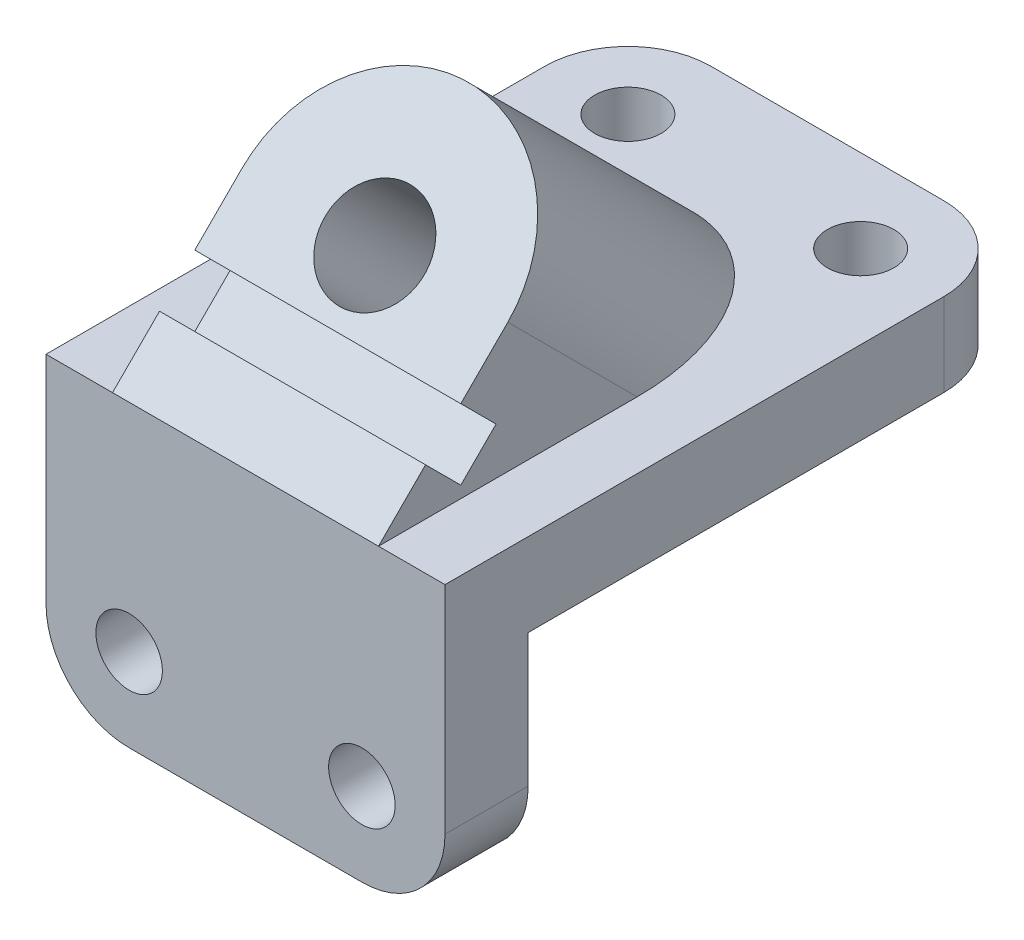
ISO-10303-21;
HEADER;
FILE_DESCRIPTION(('STEP AP214'),'2;1');
FILE_NAME('part.step','',(''),(''),'','','');
FILE_SCHEMA(('AUTOMOTIVE_DESIGN { 1 0 10303 214 1 1 1 1 }'));
ENDSEC;
DATA;
#1=APPLICATION_CONTEXT('core data for automotive mechanical design processes');
#2=APPLICATION_PROTOCOL_DEFINITION('international standard','automotive_design',2000,#1);
#3=PRODUCT_CONTEXT('',#1,'mechanical');
#4=PRODUCT('Part','Part','',(#3));
#5=PRODUCT_RELATED_PRODUCT_CATEGORY('part','',(#4));
#6=PRODUCT_DEFINITION_FORMATION('','',#4);
#7=PRODUCT_DEFINITION_CONTEXT('part definition',#1,'design');
#8=PRODUCT_DEFINITION('design','',#6,#7);
#9=PRODUCT_DEFINITION_SHAPE('','',#8);
#10=(LENGTH_UNIT() NAMED_UNIT(*) SI_UNIT(.MILLI.,.METRE.));
#11=(NAMED_UNIT(*) PLANE_ANGLE_UNIT() SI_UNIT($,.RADIAN.));
#12=(NAMED_UNIT(*) SI_UNIT($,.STERADIAN.) SOLID_ANGLE_UNIT());
#13=UNCERTAINTY_MEASURE_WITH_UNIT(LENGTH_MEASURE(1.E-05),#10,'distance_accuracy_value','');
#14=(GEOMETRIC_REPRESENTATION_CONTEXT(3) GLOBAL_UNCERTAINTY_ASSIGNED_CONTEXT((#13)) GLOBAL_UNIT_ASSIGNED_CONTEXT((#10,
#11,#12)) REPRESENTATION_CONTEXT('',''));
#15=CARTESIAN_POINT('',(0.,0.,0.));
#16=DIRECTION('',(0.,0.,1.));
#17=DIRECTION('',(1.,0.,0.));
#18=AXIS2_PLACEMENT_3D('',#15,#16,#17);
#19=CARTESIAN_POINT('',(60.,0.,0.));
#20=DIRECTION('',(0.,-0.707106781186543,-0.707106781186552));
#21=DIRECTION('',(0.,0.707106781186552,-0.707106781186543));
#22=AXIS2_PLACEMENT_3D('',#19,#20,#21);
#23=PLANE('',#22);
#24=CARTESIAN_POINT('',(0.,38.8908729652603,-38.8908729652599));
#25=DIRECTION('',(0.,0.707106781186543,0.707106781186552));
#26=DIRECTION('',(0.,-0.707106781186552,0.707106781186543));
#27=AXIS2_PLACEMENT_3D('',#24,#25,#26);
#28=CIRCLE('',#27,15.);
#29=CARTESIAN_POINT('',(0.,28.2842712474621,-28.2842712474617));
#30=VERTEX_POINT('',#29);
#31=EDGE_CURVE('E209',#30,#30,#28,.T.);
#32=ORIENTED_EDGE('',*,*,#31,.F.);
#33=EDGE_LOOP('',(#32));
#34=FACE_BOUND('',#33,.T.);
#35=DIRECTION('',(1.,0.,0.));
#36=VECTOR('',#35,1.);
#37=CARTESIAN_POINT('',(-40.,24.7487373415293,-24.748737341529));
#38=LINE('',#37,#36);
#39=CARTESIAN_POINT('',(-40.,24.7487373415293,-24.748737341529));
#40=VERTEX_POINT('',#39);
#41=CARTESIAN_POINT('',(40.,24.7487373415293,-24.748737341529));
#42=VERTEX_POINT('',#41);
#43=EDGE_CURVE('E207',#40,#42,#38,.T.);
#44=ORIENTED_EDGE('',*,*,#43,.T.);
#45=DIRECTION('',(0.,-0.707106781186552,0.707106781186543));
#46=VECTOR('',#45,1.);
#47=CARTESIAN_POINT('',(40.,0.,0.));
#48=LINE('',#47,#46);
#49=CARTESIAN_POINT('',(40.,38.8908729652603,-38.8908729652599));
#50=VERTEX_POINT('',#49);
#51=EDGE_CURVE('E243',#50,#42,#48,.T.);
#52=ORIENTED_EDGE('',*,*,#51,.F.);
#53=CARTESIAN_POINT('',(0.,38.8908729652603,-38.8908729652599));
#54=DIRECTION('',(0.,0.707106781186543,0.707106781186552));
#55=DIRECTION('',(0.,-0.707106781186552,0.707106781186543));
#56=AXIS2_PLACEMENT_3D('',#53,#54,#55);
#57=CIRCLE('',#56,40.);
#58=CARTESIAN_POINT('',(-40.,38.8908729652603,-38.8908729652599));
#59=VERTEX_POINT('',#58);
#60=EDGE_CURVE('E259',#59,#50,#57,.F.);
#61=ORIENTED_EDGE('',*,*,#60,.F.);
#62=DIRECTION('',(0.,0.707106781186552,-0.707106781186543));
#63=VECTOR('',#62,1.);
#64=CARTESIAN_POINT('',(-40.,0.,0.));
#65=LINE('',#64,#63);
#66=EDGE_CURVE('E246',#40,#59,#65,.T.);
#67=ORIENTED_EDGE('',*,*,#66,.F.);
#68=EDGE_LOOP('',(#44,#52,#61,#67));
#69=FACE_BOUND('',#68,.T.);
#70=ADVANCED_FACE('F67',(#34,#69),#23,.F.);
#71=CARTESIAN_POINT('',(-40.,-129.493706197148,-129.49370619715));
#72=DIRECTION('',(1.,0.,0.));
#73=DIRECTION('',(0.,0.,-1.));
#74=AXIS2_PLACEMENT_3D('',#71,#72,#73);
#75=PLANE('',#74);
#76=DIRECTION('',(0.,0.707106781186543,0.707106781186552));
#77=VECTOR('',#76,1.);
#78=CARTESIAN_POINT('',(-40.,14.1421356237312,-35.3553390593273));
#79=LINE('',#78,#77);
#80=CARTESIAN_POINT('',(-40.,14.1421356237312,-35.3553390593273));
#81=VERTEX_POINT('',#80);
#82=EDGE_CURVE('E202',#81,#40,#79,.T.);
#83=ORIENTED_EDGE('',*,*,#82,.T.);
#84=ORIENTED_EDGE('',*,*,#66,.T.);
#85=DIRECTION('',(0.,0.707106781186543,0.707106781186552));
#86=VECTOR('',#85,1.);
#87=CARTESIAN_POINT('',(-40.,-90.602833231888,-168.38457916241));
#88=LINE('',#87,#86);
#89=CARTESIAN_POINT('',(-40.,0.,-77.7817459305207));
#90=VERTEX_POINT('',#89);
#91=EDGE_CURVE('E253',#90,#59,#88,.T.);
#92=ORIENTED_EDGE('',*,*,#91,.F.);
#93=DIRECTION('',(0.,0.,1.));
#94=VECTOR('',#93,1.);
#95=CARTESIAN_POINT('',(-40.,0.,-129.49370619715));
#96=LINE('',#95,#94);
#97=CARTESIAN_POINT('',(-40.,0.,0.));
#98=VERTEX_POINT('',#97);
#99=EDGE_CURVE('E255',#90,#98,#96,.T.);
#100=ORIENTED_EDGE('',*,*,#99,.T.);
#101=CARTESIAN_POINT('',(-40.,14.1421356237311,-14.1421356237309));
#102=VERTEX_POINT('',#101);
#103=EDGE_CURVE('E257',#98,#102,#65,.T.);
#104=ORIENTED_EDGE('',*,*,#103,.T.);
#105=DIRECTION('',(0.,0.707106781186543,0.707106781186552));
#106=VECTOR('',#105,1.);
#107=CARTESIAN_POINT('',(-40.,3.5355339059329,-24.7487373415292));
#108=LINE('',#107,#106);
#109=CARTESIAN_POINT('',(-40.,3.5355339059329,-24.7487373415292));
#110=VERTEX_POINT('',#109);
#111=EDGE_CURVE('E213',#110,#102,#108,.T.);
#112=ORIENTED_EDGE('',*,*,#111,.F.);
#113=DIRECTION('',(0.,0.707106781186552,-0.707106781186543));
#114=VECTOR('',#113,1.);
#115=CARTESIAN_POINT('',(-40.,3.5355339059329,-24.7487373415292));
#116=LINE('',#115,#114);
#117=EDGE_CURVE('E193',#110,#81,#116,.T.);
#118=ORIENTED_EDGE('',*,*,#117,.T.);
#119=EDGE_LOOP('',(#83,#84,#92,#100,#104,#112,#118));
#120=FACE_BOUND('',#119,.T.);
#121=ADVANCED_FACE('F214',(#120),#75,.F.);
#122=CARTESIAN_POINT('',(40.,-129.493706197148,-129.49370619715));
#123=DIRECTION('',(-1.,0.,0.));
#124=DIRECTION('',(0.,-1.,0.));
#125=AXIS2_PLACEMENT_3D('',#122,#123,#124);
#126=PLANE('',#125);
#127=DIRECTION('',(0.,0.707106781186543,0.707106781186552));
#128=VECTOR('',#127,1.);
#129=CARTESIAN_POINT('',(40.,14.1421356237312,-35.3553390593273));
#130=LINE('',#129,#128);
#131=CARTESIAN_POINT('',(40.,14.1421356237312,-35.3553390593273));
#132=VERTEX_POINT('',#131);
#133=EDGE_CURVE('E208',#132,#42,#130,.T.);
#134=ORIENTED_EDGE('',*,*,#133,.F.);
#135=DIRECTION('',(0.,0.707106781186552,-0.707106781186543));
#136=VECTOR('',#135,1.);
#137=CARTESIAN_POINT('',(40.,3.5355339059329,-24.7487373415292));
#138=LINE('',#137,#136);
#139=CARTESIAN_POINT('',(40.,3.5355339059329,-24.7487373415292));
#140=VERTEX_POINT('',#139);
#141=EDGE_CURVE('E198',#140,#132,#138,.T.);
#142=ORIENTED_EDGE('',*,*,#141,.F.);
#143=DIRECTION('',(0.,0.707106781186543,0.707106781186552));
#144=VECTOR('',#143,1.);
#145=CARTESIAN_POINT('',(40.,3.5355339059329,-24.7487373415292));
#146=LINE('',#145,#144);
#147=CARTESIAN_POINT('',(40.,14.142135623731,-14.1421356237309));
#148=VERTEX_POINT('',#147);
#149=EDGE_CURVE('E230',#140,#148,#146,.T.);
#150=ORIENTED_EDGE('',*,*,#149,.T.);
#151=CARTESIAN_POINT('',(40.,0.,0.));
#152=VERTEX_POINT('',#151);
#153=EDGE_CURVE('E245',#148,#152,#48,.T.);
#154=ORIENTED_EDGE('',*,*,#153,.T.);
#155=DIRECTION('',(0.,0.,-1.));
#156=VECTOR('',#155,1.);
#157=CARTESIAN_POINT('',(40.,0.,-129.49370619715));
#158=LINE('',#157,#156);
#159=CARTESIAN_POINT('',(40.,0.,-77.7817459305207));
#160=VERTEX_POINT('',#159);
#161=EDGE_CURVE('E238',#152,#160,#158,.T.);
#162=ORIENTED_EDGE('',*,*,#161,.T.);
#163=DIRECTION('',(0.,0.707106781186543,0.707106781186552));
#164=VECTOR('',#163,1.);
#165=CARTESIAN_POINT('',(40.,-90.602833231888,-168.38457916241));
#166=LINE('',#165,#164);
#167=EDGE_CURVE('E237',#160,#50,#166,.T.);
#168=ORIENTED_EDGE('',*,*,#167,.T.);
#169=ORIENTED_EDGE('',*,*,#51,.T.);
#170=EDGE_LOOP('',(#134,#142,#150,#154,#162,#168,#169));
#171=FACE_BOUND('',#170,.T.);
#172=ADVANCED_FACE('F380',(#171),#126,.F.);
#173=CARTESIAN_POINT('',(60.,-64.9999999999998,-25.));
#174=DIRECTION('',(1.,0.,0.));
#175=DIRECTION('',(0.,1.,0.));
#176=AXIS2_PLACEMENT_3D('',#173,#174,#175);
#177=PLANE('',#176);
#178=DIRECTION('',(0.,0.,-1.));
#179=VECTOR('',#178,1.);
#180=CARTESIAN_POINT('',(60.,-25.,-175.));
#181=LINE('',#180,#179);
#182=CARTESIAN_POINT('',(60.,-25.,-25.));
#183=VERTEX_POINT('',#182);
#184=CARTESIAN_POINT('',(60.,-25.,-150.));
#185=VERTEX_POINT('',#184);
#186=EDGE_CURVE('E280',#183,#185,#181,.T.);
#187=ORIENTED_EDGE('',*,*,#186,.T.);
#188=DIRECTION('',(0.,1.,0.));
#189=VECTOR('',#188,1.);
#190=CARTESIAN_POINT('',(60.,0.,-150.));
#191=LINE('',#190,#189);
#192=CARTESIAN_POINT('',(60.,0.,-150.));
#193=VERTEX_POINT('',#192);
#194=EDGE_CURVE('E12',#185,#193,#191,.T.);
#195=ORIENTED_EDGE('',*,*,#194,.T.);
#196=DIRECTION('',(0.,0.,1.));
#197=VECTOR('',#196,1.);
#198=CARTESIAN_POINT('',(60.,0.,-25.));
#199=LINE('',#198,#197);
#200=CARTESIAN_POINT('',(60.,0.,0.));
#201=VERTEX_POINT('',#200);
#202=EDGE_CURVE('E304',#193,#201,#199,.T.);
#203=ORIENTED_EDGE('',*,*,#202,.T.);
#204=DIRECTION('',(0.,1.,0.));
#205=VECTOR('',#204,1.);
#206=CARTESIAN_POINT('',(60.,-64.9999999999998,0.));
#207=LINE('',#206,#205);
#208=CARTESIAN_POINT('',(60.,-65.,0.));
#209=VERTEX_POINT('',#208);
#210=EDGE_CURVE('E290',#209,#201,#207,.T.);
#211=ORIENTED_EDGE('',*,*,#210,.F.);
#212=DIRECTION('',(0.,0.,1.));
#213=VECTOR('',#212,1.);
#214=CARTESIAN_POINT('',(60.,-65.,-25.));
#215=LINE('',#214,#213);
#216=CARTESIAN_POINT('',(60.,-65.,-25.));
#217=VERTEX_POINT('',#216);
#218=EDGE_CURVE('E324',#217,#209,#215,.T.);
#219=ORIENTED_EDGE('',*,*,#218,.F.);
#220=DIRECTION('',(0.,1.,0.));
#221=VECTOR('',#220,1.);
#222=CARTESIAN_POINT('',(60.,-64.9999999999998,-25.));
#223=LINE('',#222,#221);
#224=EDGE_CURVE('E286',#217,#183,#223,.T.);
#225=ORIENTED_EDGE('',*,*,#224,.T.);
#226=EDGE_LOOP('',(#187,#195,#203,#211,#219,#225));
#227=FACE_BOUND('',#226,.T.);
#228=ADVANCED_FACE('F381',(#227),#177,.T.);
#229=CARTESIAN_POINT('',(-60.,-64.9999999999998,-25.));
#230=DIRECTION('',(-1.,0.,0.));
#231=DIRECTION('',(0.,0.,1.));
#232=AXIS2_PLACEMENT_3D('',#229,#230,#231);
#233=PLANE('',#232);
#234=DIRECTION('',(0.,0.,1.));
#235=VECTOR('',#234,1.);
#236=CARTESIAN_POINT('',(-60.,0.,-25.));
#237=LINE('',#236,#235);
#238=CARTESIAN_POINT('',(-60.,0.,-150.));
#239=VERTEX_POINT('',#238);
#240=CARTESIAN_POINT('',(-60.,0.,0.));
#241=VERTEX_POINT('',#240);
#242=EDGE_CURVE('E334',#239,#241,#237,.T.);
#243=ORIENTED_EDGE('',*,*,#242,.F.);
#244=DIRECTION('',(0.,1.,0.));
#245=VECTOR('',#244,1.);
#246=CARTESIAN_POINT('',(-60.,-25.,-150.));
#247=LINE('',#246,#245);
#248=CARTESIAN_POINT('',(-60.,-25.,-150.));
#249=VERTEX_POINT('',#248);
#250=EDGE_CURVE('E94',#239,#249,#247,.F.);
#251=ORIENTED_EDGE('',*,*,#250,.T.);
#252=DIRECTION('',(0.,0.,-1.));
#253=VECTOR('',#252,1.);
#254=CARTESIAN_POINT('',(-60.,-25.,-175.));
#255=LINE('',#254,#253);
#256=CARTESIAN_POINT('',(-60.,-25.,-25.));
#257=VERTEX_POINT('',#256);
#258=EDGE_CURVE('E267',#257,#249,#255,.T.);
#259=ORIENTED_EDGE('',*,*,#258,.F.);
#260=DIRECTION('',(0.,-1.,0.));
#261=VECTOR('',#260,1.);
#262=CARTESIAN_POINT('',(-60.,-64.9999999999998,-25.));
#263=LINE('',#262,#261);
#264=CARTESIAN_POINT('',(-60.,-64.9999999999998,-25.));
#265=VERTEX_POINT('',#264);
#266=EDGE_CURVE('E291',#257,#265,#263,.T.);
#267=ORIENTED_EDGE('',*,*,#266,.T.);
#268=DIRECTION('',(0.,0.,1.));
#269=VECTOR('',#268,1.);
#270=CARTESIAN_POINT('',(-60.,-64.9999999999998,-25.));
#271=LINE('',#270,#269);
#272=CARTESIAN_POINT('',(-60.,-64.9999999999998,0.));
#273=VERTEX_POINT('',#272);
#274=EDGE_CURVE('E329',#265,#273,#271,.T.);
#275=ORIENTED_EDGE('',*,*,#274,.T.);
#276=DIRECTION('',(0.,-1.,0.));
#277=VECTOR('',#276,1.);
#278=CARTESIAN_POINT('',(-60.,-64.9999999999998,0.));
#279=LINE('',#278,#277);
#280=EDGE_CURVE('E315',#241,#273,#279,.T.);
#281=ORIENTED_EDGE('',*,*,#280,.F.);
#282=EDGE_LOOP('',(#243,#251,#259,#267,#275,#281));
#283=FACE_BOUND('',#282,.T.);
#284=ADVANCED_FACE('F357',(#283),#233,.T.);
#285=CARTESIAN_POINT('',(35.,-65.,-25.));
#286=DIRECTION('',(0.,0.,1.));
#287=DIRECTION('',(1.,0.,0.));
#288=AXIS2_PLACEMENT_3D('',#285,#286,#287);
#289=CYLINDRICAL_SURFACE('',#288,25.);
#290=CARTESIAN_POINT('',(35.,-65.,0.));
#291=DIRECTION('',(0.,0.,1.));
#292=DIRECTION('',(1.,0.,0.));
#293=AXIS2_PLACEMENT_3D('',#290,#291,#292);
#294=CIRCLE('',#293,25.);
#295=CARTESIAN_POINT('',(34.9999999999999,-90.,0.));
#296=VERTEX_POINT('',#295);
#297=EDGE_CURVE('E295',#296,#209,#294,.T.);
#298=ORIENTED_EDGE('',*,*,#297,.F.);
#299=DIRECTION('',(0.,0.,1.));
#300=VECTOR('',#299,1.);
#301=CARTESIAN_POINT('',(34.9999999999999,-90.,-25.));
#302=LINE('',#301,#300);
#303=CARTESIAN_POINT('',(34.9999999999999,-90.,-25.));
#304=VERTEX_POINT('',#303);
#305=EDGE_CURVE('E326',#304,#296,#302,.T.);
#306=ORIENTED_EDGE('',*,*,#305,.F.);
#307=CARTESIAN_POINT('',(35.,-65.,-25.));
#308=DIRECTION('',(0.,0.,1.));
#309=DIRECTION('',(1.,0.,0.));
#310=AXIS2_PLACEMENT_3D('',#307,#308,#309);
#311=CIRCLE('',#310,25.);
#312=EDGE_CURVE('E305',#304,#217,#311,.T.);
#313=ORIENTED_EDGE('',*,*,#312,.T.);
#314=ORIENTED_EDGE('',*,*,#218,.T.);
#315=EDGE_LOOP('',(#298,#306,#313,#314));
#316=FACE_BOUND('',#315,.T.);
#317=ADVANCED_FACE('F439',(#316),#289,.T.);
#318=CARTESIAN_POINT('',(-34.9999999999998,-90.,-25.));
#319=DIRECTION('',(0.,-1.,0.));
#320=DIRECTION('',(1.,0.,0.));
#321=AXIS2_PLACEMENT_3D('',#318,#319,#320);
#322=PLANE('',#321);
#323=DIRECTION('',(1.,0.,0.));
#324=VECTOR('',#323,1.);
#325=CARTESIAN_POINT('',(-34.9999999999998,-90.,0.));
#326=LINE('',#325,#324);
#327=CARTESIAN_POINT('',(-34.9999999999998,-90.,0.));
#328=VERTEX_POINT('',#327);
#329=EDGE_CURVE('E319',#328,#296,#326,.T.);
#330=ORIENTED_EDGE('',*,*,#329,.F.);
#331=DIRECTION('',(0.,0.,1.));
#332=VECTOR('',#331,1.);
#333=CARTESIAN_POINT('',(-34.9999999999998,-90.,-25.));
#334=LINE('',#333,#332);
#335=CARTESIAN_POINT('',(-34.9999999999998,-90.,-25.));
#336=VERTEX_POINT('',#335);
#337=EDGE_CURVE('E328',#336,#328,#334,.T.);
#338=ORIENTED_EDGE('',*,*,#337,.F.);
#339=DIRECTION('',(1.,0.,0.));
#340=VECTOR('',#339,1.);
#341=CARTESIAN_POINT('',(-34.9999999999998,-90.,-25.));
#342=LINE('',#341,#340);
#343=EDGE_CURVE('E299',#336,#304,#342,.T.);
#344=ORIENTED_EDGE('',*,*,#343,.T.);
#345=ORIENTED_EDGE('',*,*,#305,.T.);
#346=EDGE_LOOP('',(#330,#338,#344,#345));
#347=FACE_BOUND('',#346,.T.);
#348=ADVANCED_FACE('F442',(#347),#322,.T.);
#349=CARTESIAN_POINT('',(-35.,-65.,-25.));
#350=DIRECTION('',(0.,0.,1.));
#351=DIRECTION('',(1.,0.,0.));
#352=AXIS2_PLACEMENT_3D('',#349,#350,#351);
#353=CYLINDRICAL_SURFACE('',#352,25.);
#354=CARTESIAN_POINT('',(-35.,-65.,0.));
#355=DIRECTION('',(0.,0.,1.));
#356=DIRECTION('',(-1.,0.,0.));
#357=AXIS2_PLACEMENT_3D('',#354,#355,#356);
#358=CIRCLE('',#357,25.);
#359=EDGE_CURVE('E314',#273,#328,#358,.T.);
#360=ORIENTED_EDGE('',*,*,#359,.F.);
#361=ORIENTED_EDGE('',*,*,#274,.F.);
#362=CARTESIAN_POINT('',(-35.,-65.,-25.));
#363=DIRECTION('',(0.,0.,1.));
#364=DIRECTION('',(-1.,0.,0.));
#365=AXIS2_PLACEMENT_3D('',#362,#363,#364);
#366=CIRCLE('',#365,25.);
#367=EDGE_CURVE('E298',#265,#336,#366,.T.);
#368=ORIENTED_EDGE('',*,*,#367,.T.);
#369=ORIENTED_EDGE('',*,*,#337,.T.);
#370=EDGE_LOOP('',(#360,#361,#368,#369));
#371=FACE_BOUND('',#370,.T.);
#372=ADVANCED_FACE('F450',(#371),#353,.T.);
#373=CARTESIAN_POINT('',(-60.,0.,-25.));
#374=DIRECTION('',(0.,1.,0.));
#375=DIRECTION('',(-1.,0.,0.));
#376=AXIS2_PLACEMENT_3D('',#373,#374,#375);
#377=PLANE('',#376);
#378=CARTESIAN_POINT('',(-35.,0.,-150.));
#379=DIRECTION('',(0.,1.,0.));
#380=DIRECTION('',(-1.,0.,0.));
#381=AXIS2_PLACEMENT_3D('',#378,#379,#380);
#382=CIRCLE('',#381,10.);
#383=CARTESIAN_POINT('',(-45.,0.,-150.));
#384=VERTEX_POINT('',#383);
#385=EDGE_CURVE('E477',#384,#384,#382,.T.);
#386=ORIENTED_EDGE('',*,*,#385,.F.);
#387=EDGE_LOOP('',(#386));
#388=FACE_BOUND('',#387,.T.);
#389=CARTESIAN_POINT('',(35.,0.,-150.));
#390=DIRECTION('',(0.,1.,0.));
#391=DIRECTION('',(-1.,0.,0.));
#392=AXIS2_PLACEMENT_3D('',#389,#390,#391);
#393=CIRCLE('',#392,10.);
#394=CARTESIAN_POINT('',(25.,0.,-150.));
#395=VERTEX_POINT('',#394);
#396=EDGE_CURVE('E485',#395,#395,#393,.T.);
#397=ORIENTED_EDGE('',*,*,#396,.F.);
#398=EDGE_LOOP('',(#397));
#399=FACE_BOUND('',#398,.T.);
#400=DIRECTION('',(-1.,0.,0.));
#401=VECTOR('',#400,1.);
#402=CARTESIAN_POINT('',(60.,0.,-175.));
#403=LINE('',#402,#401);
#404=CARTESIAN_POINT('',(35.,0.,-175.));
#405=VERTEX_POINT('',#404);
#406=CARTESIAN_POINT('',(-35.,0.,-175.));
#407=VERTEX_POINT('',#406);
#408=EDGE_CURVE('E276',#405,#407,#403,.T.);
#409=ORIENTED_EDGE('',*,*,#408,.T.);
#410=CARTESIAN_POINT('',(-35.,0.,-150.));
#411=DIRECTION('',(0.,1.,0.));
#412=DIRECTION('',(-1.,0.,0.));
#413=AXIS2_PLACEMENT_3D('',#410,#411,#412);
#414=CIRCLE('',#413,25.);
#415=EDGE_CURVE('E342',#407,#239,#414,.T.);
#416=ORIENTED_EDGE('',*,*,#415,.T.);
#417=ORIENTED_EDGE('',*,*,#242,.T.);
#418=DIRECTION('',(1.,0.,0.));
#419=VECTOR('',#418,1.);
#420=CARTESIAN_POINT('',(0.,0.,0.));
#421=LINE('',#420,#419);
#422=EDGE_CURVE('E258',#241,#98,#421,.T.);
#423=ORIENTED_EDGE('',*,*,#422,.T.);
#424=ORIENTED_EDGE('',*,*,#99,.F.);
#425=CARTESIAN_POINT('',(0.,0.,-77.7817459305207));
#426=DIRECTION('',(0.,1.,0.));
#427=DIRECTION('',(0.,0.,1.));
#428=AXIS2_PLACEMENT_3D('',#425,#426,#427);
#429=ELLIPSE('',#428,56.5685424949241,40.);
#430=EDGE_CURVE('E248',#160,#90,#429,.T.);
#431=ORIENTED_EDGE('',*,*,#430,.F.);
#432=ORIENTED_EDGE('',*,*,#161,.F.);
#433=DIRECTION('',(-1.,0.,0.));
#434=VECTOR('',#433,1.);
#435=CARTESIAN_POINT('',(-60.,0.,0.));
#436=LINE('',#435,#434);
#437=EDGE_CURVE('E307',#201,#152,#436,.T.);
#438=ORIENTED_EDGE('',*,*,#437,.F.);
#439=ORIENTED_EDGE('',*,*,#202,.F.);
#440=CARTESIAN_POINT('',(35.,0.,-150.));
#441=DIRECTION('',(0.,1.,0.));
#442=DIRECTION('',(-1.,0.,0.));
#443=AXIS2_PLACEMENT_3D('',#440,#441,#442);
#444=CIRCLE('',#443,25.);
#445=EDGE_CURVE('E339',#193,#405,#444,.T.);
#446=ORIENTED_EDGE('',*,*,#445,.T.);
#447=EDGE_LOOP('',(#409,#416,#417,#423,#424,#431,#432,#438,#439,#446));
#448=FACE_BOUND('',#447,.T.);
#449=ADVANCED_FACE('F355',(#388,#399,#448),#377,.T.);
#450=CARTESIAN_POINT('',(-35.,-65.,-25.));
#451=DIRECTION('',(0.,0.,-1.));
#452=DIRECTION('',(-1.,0.,0.));
#453=AXIS2_PLACEMENT_3D('',#450,#451,#452);
#454=PLANE('',#453);
#455=CARTESIAN_POINT('',(-35.,-65.,-25.));
#456=DIRECTION('',(0.,0.,-1.));
#457=DIRECTION('',(-1.,0.,0.));
#458=AXIS2_PLACEMENT_3D('',#455,#456,#457);
#459=CIRCLE('',#458,10.);
#460=CARTESIAN_POINT('',(-45.,-65.,-25.));
#461=VERTEX_POINT('',#460);
#462=EDGE_CURVE('E270',#461,#461,#459,.F.);
#463=ORIENTED_EDGE('',*,*,#462,.T.);
#464=EDGE_LOOP('',(#463));
#465=FACE_BOUND('',#464,.T.);
#466=CARTESIAN_POINT('',(35.,-65.,-25.));
#467=DIRECTION('',(0.,0.,-1.));
#468=DIRECTION('',(-1.,0.,0.));
#469=AXIS2_PLACEMENT_3D('',#466,#467,#468);
#470=CIRCLE('',#469,10.);
#471=CARTESIAN_POINT('',(25.,-65.,-25.));
#472=VERTEX_POINT('',#471);
#473=EDGE_CURVE('E252',#472,#472,#470,.F.);
#474=ORIENTED_EDGE('',*,*,#473,.T.);
#475=EDGE_LOOP('',(#474));
#476=FACE_BOUND('',#475,.T.);
#477=DIRECTION('',(-1.,0.,0.));
#478=VECTOR('',#477,1.);
#479=CARTESIAN_POINT('',(60.,-25.,-25.));
#480=LINE('',#479,#478);
#481=EDGE_CURVE('E288',#183,#257,#480,.T.);
#482=ORIENTED_EDGE('',*,*,#481,.F.);
#483=ORIENTED_EDGE('',*,*,#224,.F.);
#484=ORIENTED_EDGE('',*,*,#312,.F.);
#485=ORIENTED_EDGE('',*,*,#343,.F.);
#486=ORIENTED_EDGE('',*,*,#367,.F.);
#487=ORIENTED_EDGE('',*,*,#266,.F.);
#488=EDGE_LOOP('',(#482,#483,#484,#485,#486,#487));
#489=FACE_BOUND('',#488,.T.);
#490=ADVANCED_FACE('F432',(#465,#476,#489),#454,.T.);
#491=CARTESIAN_POINT('',(-35.,-65.,0.));
#492=DIRECTION('',(0.,0.,-1.));
#493=DIRECTION('',(-1.,0.,0.));
#494=AXIS2_PLACEMENT_3D('',#491,#492,#493);
#495=PLANE('',#494);
#496=CARTESIAN_POINT('',(-35.,-65.,0.));
#497=DIRECTION('',(0.,0.,1.));
#498=DIRECTION('',(1.,0.,0.));
#499=AXIS2_PLACEMENT_3D('',#496,#497,#498);
#500=CIRCLE('',#499,10.);
#501=CARTESIAN_POINT('',(-25.,-65.,0.));
#502=VERTEX_POINT('',#501);
#503=EDGE_CURVE('E264',#502,#502,#500,.T.);
#504=ORIENTED_EDGE('',*,*,#503,.F.);
#505=EDGE_LOOP('',(#504));
#506=FACE_BOUND('',#505,.T.);
#507=CARTESIAN_POINT('',(35.,-65.,0.));
#508=DIRECTION('',(0.,0.,1.));
#509=DIRECTION('',(1.,0.,0.));
#510=AXIS2_PLACEMENT_3D('',#507,#508,#509);
#511=CIRCLE('',#510,10.);
#512=CARTESIAN_POINT('',(45.,-65.,0.));
#513=VERTEX_POINT('',#512);
#514=EDGE_CURVE('E275',#513,#513,#511,.T.);
#515=ORIENTED_EDGE('',*,*,#514,.F.);
#516=EDGE_LOOP('',(#515));
#517=FACE_BOUND('',#516,.T.);
#518=ORIENTED_EDGE('',*,*,#210,.T.);
#519=ORIENTED_EDGE('',*,*,#437,.T.);
#520=EDGE_CURVE('E308',#152,#98,#436,.T.);
#521=ORIENTED_EDGE('',*,*,#520,.T.);
#522=ORIENTED_EDGE('',*,*,#422,.F.);
#523=ORIENTED_EDGE('',*,*,#280,.T.);
#524=ORIENTED_EDGE('',*,*,#359,.T.);
#525=ORIENTED_EDGE('',*,*,#329,.T.);
#526=ORIENTED_EDGE('',*,*,#297,.T.);
#527=EDGE_LOOP('',(#518,#519,#521,#522,#523,#524,#525,#526));
#528=FACE_BOUND('',#527,.T.);
#529=ADVANCED_FACE('F363',(#506,#517,#528),#495,.F.);
#530=CARTESIAN_POINT('',(60.,-25.,-175.));
#531=DIRECTION('',(0.,1.,0.));
#532=DIRECTION('',(0.,0.,1.));
#533=AXIS2_PLACEMENT_3D('',#530,#531,#532);
#534=PLANE('',#533);
#535=CARTESIAN_POINT('',(-35.,-25.,-150.));
#536=DIRECTION('',(0.,1.,0.));
#537=DIRECTION('',(0.,0.,1.));
#538=AXIS2_PLACEMENT_3D('',#535,#536,#537);
#539=CIRCLE('',#538,10.);
#540=CARTESIAN_POINT('',(-45.,-25.,-150.));
#541=VERTEX_POINT('',#540);
#542=EDGE_CURVE('E228',#541,#541,#539,.F.);
#543=ORIENTED_EDGE('',*,*,#542,.F.);
#544=EDGE_LOOP('',(#543));
#545=FACE_BOUND('',#544,.T.);
#546=CARTESIAN_POINT('',(35.,-25.,-150.));
#547=DIRECTION('',(0.,1.,0.));
#548=DIRECTION('',(0.,0.,1.));
#549=AXIS2_PLACEMENT_3D('',#546,#547,#548);
#550=CIRCLE('',#549,10.);
#551=CARTESIAN_POINT('',(25.,-25.,-150.));
#552=VERTEX_POINT('',#551);
#553=EDGE_CURVE('E219',#552,#552,#550,.F.);
#554=ORIENTED_EDGE('',*,*,#553,.F.);
#555=EDGE_LOOP('',(#554));
#556=FACE_BOUND('',#555,.T.);
#557=CARTESIAN_POINT('',(0.,-25.,-102.781745930521));
#558=DIRECTION('',(0.,1.,0.));
#559=DIRECTION('',(0.,0.,1.));
#560=AXIS2_PLACEMENT_3D('',#557,#558,#559);
#561=ELLIPSE('',#560,21.2132034355965,15.);
#562=CARTESIAN_POINT('',(0.,-25.,-81.5685424949245));
#563=VERTEX_POINT('',#562);
#564=EDGE_CURVE('E232',#563,#563,#561,.F.);
#565=ORIENTED_EDGE('',*,*,#564,.F.);
#566=EDGE_LOOP('',(#565));
#567=FACE_BOUND('',#566,.T.);
#568=ORIENTED_EDGE('',*,*,#258,.T.);
#569=CARTESIAN_POINT('',(-35.,-25.,-150.));
#570=DIRECTION('',(0.,1.,0.));
#571=DIRECTION('',(0.,0.,1.));
#572=AXIS2_PLACEMENT_3D('',#569,#570,#571);
#573=CIRCLE('',#572,25.);
#574=CARTESIAN_POINT('',(-35.,-25.,-175.));
#575=VERTEX_POINT('',#574);
#576=EDGE_CURVE('E80',#249,#575,#573,.F.);
#577=ORIENTED_EDGE('',*,*,#576,.T.);
#578=DIRECTION('',(-1.,0.,0.));
#579=VECTOR('',#578,1.);
#580=CARTESIAN_POINT('',(60.,-25.,-175.));
#581=LINE('',#580,#579);
#582=CARTESIAN_POINT('',(35.,-25.,-175.));
#583=VERTEX_POINT('',#582);
#584=EDGE_CURVE('E283',#583,#575,#581,.T.);
#585=ORIENTED_EDGE('',*,*,#584,.F.);
#586=CARTESIAN_POINT('',(35.,-25.,-150.));
#587=DIRECTION('',(0.,1.,0.));
#588=DIRECTION('',(0.,0.,1.));
#589=AXIS2_PLACEMENT_3D('',#586,#587,#588);
#590=CIRCLE('',#589,25.);
#591=EDGE_CURVE('E81',#583,#185,#590,.F.);
#592=ORIENTED_EDGE('',*,*,#591,.T.);
#593=ORIENTED_EDGE('',*,*,#186,.F.);
#594=ORIENTED_EDGE('',*,*,#481,.T.);
#595=EDGE_LOOP('',(#568,#577,#585,#592,#593,#594));
#596=FACE_BOUND('',#595,.T.);
#597=ADVANCED_FACE('F343',(#545,#556,#567,#596),#534,.F.);
#598=CARTESIAN_POINT('',(60.,0.,-175.));
#599=DIRECTION('',(0.,0.,1.));
#600=DIRECTION('',(1.,0.,0.));
#601=AXIS2_PLACEMENT_3D('',#598,#599,#600);
#602=PLANE('',#601);
#603=ORIENTED_EDGE('',*,*,#584,.T.);
#604=DIRECTION('',(0.,1.,0.));
#605=VECTOR('',#604,1.);
#606=CARTESIAN_POINT('',(-35.,0.,-175.));
#607=LINE('',#606,#605);
#608=EDGE_CURVE('E337',#575,#407,#607,.T.);
#609=ORIENTED_EDGE('',*,*,#608,.T.);
#610=ORIENTED_EDGE('',*,*,#408,.F.);
#611=DIRECTION('',(0.,1.,0.));
#612=VECTOR('',#611,1.);
#613=CARTESIAN_POINT('',(35.,-25.,-175.));
#614=LINE('',#613,#612);
#615=EDGE_CURVE('E323',#405,#583,#614,.F.);
#616=ORIENTED_EDGE('',*,*,#615,.T.);
#617=EDGE_LOOP('',(#603,#609,#610,#616));
#618=FACE_BOUND('',#617,.T.);
#619=ADVANCED_FACE('F347',(#618),#602,.F.);
#620=CARTESIAN_POINT('',(35.,-65.,-175.001));
#621=DIRECTION('',(0.,0.,1.));
#622=DIRECTION('',(1.,0.,0.));
#623=AXIS2_PLACEMENT_3D('',#620,#621,#622);
#624=CYLINDRICAL_SURFACE('',#623,10.);
#625=ORIENTED_EDGE('',*,*,#473,.F.);
#626=EDGE_LOOP('',(#625));
#627=FACE_BOUND('',#626,.T.);
#628=ORIENTED_EDGE('',*,*,#514,.T.);
#629=EDGE_LOOP('',(#628));
#630=FACE_BOUND('',#629,.T.);
#631=ADVANCED_FACE('F417',(#627,#630),#624,.F.);
#632=CARTESIAN_POINT('',(-35.,-65.,-175.001));
#633=DIRECTION('',(0.,0.,1.));
#634=DIRECTION('',(1.,0.,0.));
#635=AXIS2_PLACEMENT_3D('',#632,#633,#634);
#636=CYLINDRICAL_SURFACE('',#635,10.);
#637=ORIENTED_EDGE('',*,*,#462,.F.);
#638=EDGE_LOOP('',(#637));
#639=FACE_BOUND('',#638,.T.);
#640=ORIENTED_EDGE('',*,*,#503,.T.);
#641=EDGE_LOOP('',(#640));
#642=FACE_BOUND('',#641,.T.);
#643=ADVANCED_FACE('F406',(#639,#642),#636,.F.);
#644=ORIENTED_EDGE('',*,*,#153,.F.);
#645=DIRECTION('',(1.,0.,0.));
#646=VECTOR('',#645,1.);
#647=CARTESIAN_POINT('',(-40.,14.1421356237311,-14.1421356237309));
#648=LINE('',#647,#646);
#649=EDGE_CURVE('E216',#102,#148,#648,.T.);
#650=ORIENTED_EDGE('',*,*,#649,.F.);
#651=ORIENTED_EDGE('',*,*,#103,.F.);
#652=ORIENTED_EDGE('',*,*,#520,.F.);
#653=EDGE_LOOP('',(#644,#650,#651,#652));
#654=FACE_BOUND('',#653,.T.);
#655=ADVANCED_FACE('F368',(#654),#23,.F.);
#656=CARTESIAN_POINT('',(0.,-90.602833231888,-168.38457916241));
#657=DIRECTION('',(0.,0.707106781186543,0.707106781186552));
#658=DIRECTION('',(0.,-0.707106781186552,0.707106781186543));
#659=AXIS2_PLACEMENT_3D('',#656,#657,#658);
#660=CYLINDRICAL_SURFACE('',#659,40.);
#661=ORIENTED_EDGE('',*,*,#430,.T.);
#662=ORIENTED_EDGE('',*,*,#91,.T.);
#663=ORIENTED_EDGE('',*,*,#60,.T.);
#664=ORIENTED_EDGE('',*,*,#167,.F.);
#665=EDGE_LOOP('',(#661,#662,#663,#664));
#666=FACE_BOUND('',#665,.T.);
#667=ADVANCED_FACE('F375',(#666),#660,.T.);
#668=CARTESIAN_POINT('',(0.,-93.6101270347391,-171.391872965261));
#669=DIRECTION('',(0.,0.707106781186543,0.707106781186552));
#670=DIRECTION('',(0.,-0.707106781186552,0.707106781186543));
#671=AXIS2_PLACEMENT_3D('',#668,#669,#670);
#672=CYLINDRICAL_SURFACE('',#671,15.);
#673=ORIENTED_EDGE('',*,*,#31,.T.);
#674=EDGE_LOOP('',(#673));
#675=FACE_BOUND('',#674,.T.);
#676=ORIENTED_EDGE('',*,*,#564,.T.);
#677=EDGE_LOOP('',(#676));
#678=FACE_BOUND('',#677,.T.);
#679=ADVANCED_FACE('F414',(#675,#678),#672,.F.);
#680=CARTESIAN_POINT('',(-40.,14.1421356237312,-35.3553390593273));
#681=DIRECTION('',(0.,-0.707106781186552,0.707106781186543));
#682=DIRECTION('',(0.,-0.707106781186543,-0.707106781186552));
#683=AXIS2_PLACEMENT_3D('',#680,#681,#682);
#684=PLANE('',#683);
#685=ORIENTED_EDGE('',*,*,#43,.F.);
#686=ORIENTED_EDGE('',*,*,#82,.F.);
#687=DIRECTION('',(1.,0.,0.));
#688=VECTOR('',#687,1.);
#689=CARTESIAN_POINT('',(-40.,14.1421356237312,-35.3553390593273));
#690=LINE('',#689,#688);
#691=EDGE_CURVE('E192',#81,#132,#690,.T.);
#692=ORIENTED_EDGE('',*,*,#691,.T.);
#693=ORIENTED_EDGE('',*,*,#133,.T.);
#694=EDGE_LOOP('',(#685,#686,#692,#693));
#695=FACE_BOUND('',#694,.T.);
#696=ADVANCED_FACE('F205',(#695),#684,.T.);
#697=CARTESIAN_POINT('',(-40.,3.5355339059329,-24.7487373415292));
#698=DIRECTION('',(0.,-0.707106781186552,0.707106781186543));
#699=DIRECTION('',(0.,-0.707106781186543,-0.707106781186552));
#700=AXIS2_PLACEMENT_3D('',#697,#698,#699);
#701=PLANE('',#700);
#702=ORIENTED_EDGE('',*,*,#649,.T.);
#703=ORIENTED_EDGE('',*,*,#149,.F.);
#704=DIRECTION('',(1.,0.,0.));
#705=VECTOR('',#704,1.);
#706=CARTESIAN_POINT('',(-40.,3.5355339059329,-24.7487373415292));
#707=LINE('',#706,#705);
#708=EDGE_CURVE('E225',#110,#140,#707,.T.);
#709=ORIENTED_EDGE('',*,*,#708,.F.);
#710=ORIENTED_EDGE('',*,*,#111,.T.);
#711=EDGE_LOOP('',(#702,#703,#709,#710));
#712=FACE_BOUND('',#711,.T.);
#713=ADVANCED_FACE('F470',(#712),#701,.F.);
#714=CARTESIAN_POINT('',(0.,-10.6066017177982,-10.6066017177983));
#715=DIRECTION('',(0.,-0.707106781186543,-0.707106781186552));
#716=DIRECTION('',(0.,0.707106781186552,-0.707106781186543));
#717=AXIS2_PLACEMENT_3D('',#714,#715,#716);
#718=PLANE('',#717);
#719=ORIENTED_EDGE('',*,*,#117,.F.);
#720=ORIENTED_EDGE('',*,*,#708,.T.);
#721=ORIENTED_EDGE('',*,*,#141,.T.);
#722=ORIENTED_EDGE('',*,*,#691,.F.);
#723=EDGE_LOOP('',(#719,#720,#721,#722));
#724=FACE_BOUND('',#723,.T.);
#725=ADVANCED_FACE('F194',(#724),#718,.F.);
#726=CARTESIAN_POINT('',(-35.,0.,-150.));
#727=DIRECTION('',(0.,-1.,0.));
#728=DIRECTION('',(0.,0.,-1.));
#729=AXIS2_PLACEMENT_3D('',#726,#727,#728);
#730=CYLINDRICAL_SURFACE('',#729,25.);
#731=ORIENTED_EDGE('',*,*,#576,.F.);
#732=ORIENTED_EDGE('',*,*,#250,.F.);
#733=ORIENTED_EDGE('',*,*,#415,.F.);
#734=ORIENTED_EDGE('',*,*,#608,.F.);
#735=EDGE_LOOP('',(#731,#732,#733,#734));
#736=FACE_BOUND('',#735,.T.);
#737=ADVANCED_FACE('F354',(#736),#730,.T.);
#738=CARTESIAN_POINT('',(35.,-64.9999999999998,-150.));
#739=DIRECTION('',(0.,-1.,0.));
#740=DIRECTION('',(1.,0.,0.));
#741=AXIS2_PLACEMENT_3D('',#738,#739,#740);
#742=CYLINDRICAL_SURFACE('',#741,25.);
#743=ORIENTED_EDGE('',*,*,#591,.F.);
#744=ORIENTED_EDGE('',*,*,#615,.F.);
#745=ORIENTED_EDGE('',*,*,#445,.F.);
#746=ORIENTED_EDGE('',*,*,#194,.F.);
#747=EDGE_LOOP('',(#743,#744,#745,#746));
#748=FACE_BOUND('',#747,.T.);
#749=ADVANCED_FACE('F73',(#748),#742,.T.);
#750=CARTESIAN_POINT('',(35.,-90.001,-150.));
#751=DIRECTION('',(0.,1.,0.));
#752=DIRECTION('',(-1.,0.,0.));
#753=AXIS2_PLACEMENT_3D('',#750,#751,#752);
#754=CYLINDRICAL_SURFACE('',#753,10.);
#755=CARTESIAN_POINT('',(25.,0.,-150.));
#756=CARTESIAN_POINT('',(25.,-0.260416666666666,-150.));
#757=CARTESIAN_POINT('',(25.,-0.520833333333331,-150.));
#758=CARTESIAN_POINT('',(25.,-1.04166666666666,-150.));
#759=CARTESIAN_POINT('',(25.,-1.30208333333333,-150.));
#760=CARTESIAN_POINT('',(25.,-1.82291666666666,-150.));
#761=CARTESIAN_POINT('',(25.,-2.08333333333334,-150.));
#762=CARTESIAN_POINT('',(25.,-2.60416666666667,-150.));
#763=CARTESIAN_POINT('',(25.,-2.86458333333334,-150.));
#764=CARTESIAN_POINT('',(25.,-3.38541666666667,-150.));
#765=CARTESIAN_POINT('',(25.,-3.64583333333333,-150.));
#766=CARTESIAN_POINT('',(25.,-4.16666666666667,-150.));
#767=CARTESIAN_POINT('',(25.,-4.42708333333334,-150.));
#768=CARTESIAN_POINT('',(25.,-4.94791666666668,-150.));
#769=CARTESIAN_POINT('',(25.,-5.20833333333334,-150.));
#770=CARTESIAN_POINT('',(25.,-5.72916666666667,-150.));
#771=CARTESIAN_POINT('',(25.,-5.98958333333334,-150.));
#772=CARTESIAN_POINT('',(25.,-6.51041666666667,-150.));
#773=CARTESIAN_POINT('',(25.,-6.77083333333334,-150.));
#774=CARTESIAN_POINT('',(25.,-7.29166666666667,-150.));
#775=CARTESIAN_POINT('',(25.,-7.55208333333333,-150.));
#776=CARTESIAN_POINT('',(25.,-8.07291666666667,-150.));
#777=CARTESIAN_POINT('',(25.,-8.33333333333334,-150.));
#778=CARTESIAN_POINT('',(25.,-8.85416666666668,-150.));
#779=CARTESIAN_POINT('',(25.,-9.11458333333334,-150.));
#780=CARTESIAN_POINT('',(25.,-9.63541666666667,-150.));
#781=CARTESIAN_POINT('',(25.,-9.89583333333334,-150.));
#782=CARTESIAN_POINT('',(25.,-10.4166666666667,-150.));
#783=CARTESIAN_POINT('',(25.,-10.6770833333333,-150.));
#784=CARTESIAN_POINT('',(25.,-11.1979166666667,-150.));
#785=CARTESIAN_POINT('',(25.,-11.4583333333333,-150.));
#786=CARTESIAN_POINT('',(25.,-11.9791666666667,-150.));
#787=CARTESIAN_POINT('',(25.,-12.2395833333333,-150.));
#788=CARTESIAN_POINT('',(25.,-12.7604166666667,-150.));
#789=CARTESIAN_POINT('',(25.,-13.0208333333333,-150.));
#790=CARTESIAN_POINT('',(25.,-13.5416666666667,-150.));
#791=CARTESIAN_POINT('',(25.,-13.8020833333333,-150.));
#792=CARTESIAN_POINT('',(25.,-14.3229166666667,-150.));
#793=CARTESIAN_POINT('',(25.,-14.5833333333333,-150.));
#794=CARTESIAN_POINT('',(25.,-15.1041666666667,-150.));
#795=CARTESIAN_POINT('',(25.,-15.3645833333333,-150.));
#796=CARTESIAN_POINT('',(25.,-15.8854166666667,-150.));
#797=CARTESIAN_POINT('',(25.,-16.1458333333333,-150.));
#798=CARTESIAN_POINT('',(25.,-16.6666666666667,-150.));
#799=CARTESIAN_POINT('',(25.,-16.9270833333334,-150.));
#800=CARTESIAN_POINT('',(25.,-17.4479166666667,-150.));
#801=CARTESIAN_POINT('',(25.,-17.7083333333334,-150.));
#802=CARTESIAN_POINT('',(25.,-18.2291666666667,-150.));
#803=CARTESIAN_POINT('',(25.,-18.4895833333333,-150.));
#804=CARTESIAN_POINT('',(25.,-19.0104166666667,-150.));
#805=CARTESIAN_POINT('',(25.,-19.2708333333333,-150.));
#806=CARTESIAN_POINT('',(25.,-19.7916666666667,-150.));
#807=CARTESIAN_POINT('',(25.,-20.0520833333333,-150.));
#808=CARTESIAN_POINT('',(25.,-20.5729166666667,-150.));
#809=CARTESIAN_POINT('',(25.,-20.8333333333334,-150.));
#810=CARTESIAN_POINT('',(25.,-21.3541666666667,-150.));
#811=CARTESIAN_POINT('',(25.,-21.6145833333334,-150.));
#812=CARTESIAN_POINT('',(25.,-22.1354166666667,-150.));
#813=CARTESIAN_POINT('',(25.,-22.3958333333333,-150.));
#814=CARTESIAN_POINT('',(25.,-22.9166666666667,-150.));
#815=CARTESIAN_POINT('',(25.,-23.1770833333334,-150.));
#816=CARTESIAN_POINT('',(25.,-23.6979166666667,-150.));
#817=CARTESIAN_POINT('',(25.,-23.9583333333334,-150.));
#818=CARTESIAN_POINT('',(25.,-24.4791666666667,-150.));
#819=CARTESIAN_POINT('',(25.,-24.7395833333334,-150.));
#820=CARTESIAN_POINT('',(25.,-25.,-150.));
#821=B_SPLINE_CURVE_WITH_KNOTS('',3,(#755,#756,#757,#758,#759,#760,#761,#762,#763,#764,#765,
#766,#767,#768,#769,#770,#771,#772,#773,#774,#775,#776,#777,#778,#779,#780,#781,#782,#783,#784,
#785,#786,#787,#788,#789,#790,#791,#792,#793,#794,#795,#796,#797,#798,#799,#800,#801,#802,#803,
#804,#805,#806,#807,#808,#809,#810,#811,#812,#813,#814,#815,#816,#817,#818,#819,#820),
.UNSPECIFIED.,.F.,.F.,(4,2,2,2,2,2,2,2,2,2,2,2,2,2,2,2,2,2,2,2,2,2,2,2,2,2,2,2,2,2,2,2,4),(0.,
0.781249999999997,1.56249999999999,2.34375000000001,3.125,3.90625,4.68750000000001,
5.46875000000001,6.25000000000001,7.03125,7.8125,8.59375000000001,9.37500000000001,10.15625,
10.9375,11.71875,12.5,13.28125,14.0625,14.84375,15.625,16.40625,17.1875,17.96875,18.75,19.53125,
20.3125,21.09375,21.875,22.65625,23.4375,24.21875,25.),.UNSPECIFIED.);
#822=EDGE_CURVE('BSEAM386',#395,#552,#821,.T.);
#823=ORIENTED_EDGE('',*,*,#396,.T.);
#824=ORIENTED_EDGE('',*,*,#553,.T.);
#825=ORIENTED_EDGE('',*,*,#822,.T.);
#826=ORIENTED_EDGE('',*,*,#822,.F.);
#827=EDGE_LOOP('',(#823,#825,#824,#826));
#828=FACE_BOUND('',#827,.T.);
#829=ADVANCED_FACE('F386',(#828),#754,.F.);
#830=CARTESIAN_POINT('',(-35.,-90.001,-150.));
#831=DIRECTION('',(0.,1.,0.));
#832=DIRECTION('',(-1.,0.,0.));
#833=AXIS2_PLACEMENT_3D('',#830,#831,#832);
#834=CYLINDRICAL_SURFACE('',#833,10.);
#835=CARTESIAN_POINT('',(-45.,0.,-150.));
#836=CARTESIAN_POINT('',(-45.,-0.260416666666666,-150.));
#837=CARTESIAN_POINT('',(-45.,-0.520833333333331,-150.));
#838=CARTESIAN_POINT('',(-45.,-1.04166666666666,-150.));
#839=CARTESIAN_POINT('',(-45.,-1.30208333333333,-150.));
#840=CARTESIAN_POINT('',(-45.,-1.82291666666666,-150.));
#841=CARTESIAN_POINT('',(-45.,-2.08333333333334,-150.));
#842=CARTESIAN_POINT('',(-45.,-2.60416666666667,-150.));
#843=CARTESIAN_POINT('',(-45.,-2.86458333333334,-150.));
#844=CARTESIAN_POINT('',(-45.,-3.38541666666667,-150.));
#845=CARTESIAN_POINT('',(-45.,-3.64583333333333,-150.));
#846=CARTESIAN_POINT('',(-45.,-4.16666666666667,-150.));
#847=CARTESIAN_POINT('',(-45.,-4.42708333333334,-150.));
#848=CARTESIAN_POINT('',(-45.,-4.94791666666668,-150.));
#849=CARTESIAN_POINT('',(-45.,-5.20833333333334,-150.));
#850=CARTESIAN_POINT('',(-45.,-5.72916666666667,-150.));
#851=CARTESIAN_POINT('',(-45.,-5.98958333333334,-150.));
#852=CARTESIAN_POINT('',(-45.,-6.51041666666667,-150.));
#853=CARTESIAN_POINT('',(-45.,-6.77083333333334,-150.));
#854=CARTESIAN_POINT('',(-45.,-7.29166666666667,-150.));
#855=CARTESIAN_POINT('',(-45.,-7.55208333333333,-150.));
#856=CARTESIAN_POINT('',(-45.,-8.07291666666667,-150.));
#857=CARTESIAN_POINT('',(-45.,-8.33333333333334,-150.));
#858=CARTESIAN_POINT('',(-45.,-8.85416666666668,-150.));
#859=CARTESIAN_POINT('',(-45.,-9.11458333333334,-150.));
#860=CARTESIAN_POINT('',(-45.,-9.63541666666667,-150.));
#861=CARTESIAN_POINT('',(-45.,-9.89583333333334,-150.));
#862=CARTESIAN_POINT('',(-45.,-10.4166666666667,-150.));
#863=CARTESIAN_POINT('',(-45.,-10.6770833333333,-150.));
#864=CARTESIAN_POINT('',(-45.,-11.1979166666667,-150.));
#865=CARTESIAN_POINT('',(-45.,-11.4583333333333,-150.));
#866=CARTESIAN_POINT('',(-45.,-11.9791666666667,-150.));
#867=CARTESIAN_POINT('',(-45.,-12.2395833333333,-150.));
#868=CARTESIAN_POINT('',(-45.,-12.7604166666667,-150.));
#869=CARTESIAN_POINT('',(-45.,-13.0208333333333,-150.));
#870=CARTESIAN_POINT('',(-45.,-13.5416666666667,-150.));
#871=CARTESIAN_POINT('',(-45.,-13.8020833333333,-150.));
#872=CARTESIAN_POINT('',(-45.,-14.3229166666667,-150.));
#873=CARTESIAN_POINT('',(-45.,-14.5833333333333,-150.));
#874=CARTESIAN_POINT('',(-45.,-15.1041666666667,-150.));
#875=CARTESIAN_POINT('',(-45.,-15.3645833333333,-150.));
#876=CARTESIAN_POINT('',(-45.,-15.8854166666667,-150.));
#877=CARTESIAN_POINT('',(-45.,-16.1458333333333,-150.));
#878=CARTESIAN_POINT('',(-45.,-16.6666666666667,-150.));
#879=CARTESIAN_POINT('',(-45.,-16.9270833333334,-150.));
#880=CARTESIAN_POINT('',(-45.,-17.4479166666667,-150.));
#881=CARTESIAN_POINT('',(-45.,-17.7083333333334,-150.));
#882=CARTESIAN_POINT('',(-45.,-18.2291666666667,-150.));
#883=CARTESIAN_POINT('',(-45.,-18.4895833333333,-150.));
#884=CARTESIAN_POINT('',(-45.,-19.0104166666667,-150.));
#885=CARTESIAN_POINT('',(-45.,-19.2708333333333,-150.));
#886=CARTESIAN_POINT('',(-45.,-19.7916666666667,-150.));
#887=CARTESIAN_POINT('',(-45.,-20.0520833333333,-150.));
#888=CARTESIAN_POINT('',(-45.,-20.5729166666667,-150.));
#889=CARTESIAN_POINT('',(-45.,-20.8333333333334,-150.));
#890=CARTESIAN_POINT('',(-45.,-21.3541666666667,-150.));
#891=CARTESIAN_POINT('',(-45.,-21.6145833333334,-150.));
#892=CARTESIAN_POINT('',(-45.,-22.1354166666667,-150.));
#893=CARTESIAN_POINT('',(-45.,-22.3958333333333,-150.));
#894=CARTESIAN_POINT('',(-45.,-22.9166666666667,-150.));
#895=CARTESIAN_POINT('',(-45.,-23.1770833333334,-150.));
#896=CARTESIAN_POINT('',(-45.,-23.6979166666667,-150.));
#897=CARTESIAN_POINT('',(-45.,-23.9583333333334,-150.));
#898=CARTESIAN_POINT('',(-45.,-24.4791666666667,-150.));
#899=CARTESIAN_POINT('',(-45.,-24.7395833333334,-150.));
#900=CARTESIAN_POINT('',(-45.,-25.,-150.));
#901=B_SPLINE_CURVE_WITH_KNOTS('',3,(#835,#836,#837,#838,#839,#840,#841,#842,#843,#844,#845,
#846,#847,#848,#849,#850,#851,#852,#853,#854,#855,#856,#857,#858,#859,#860,#861,#862,#863,#864,
#865,#866,#867,#868,#869,#870,#871,#872,#873,#874,#875,#876,#877,#878,#879,#880,#881,#882,#883,
#884,#885,#886,#887,#888,#889,#890,#891,#892,#893,#894,#895,#896,#897,#898,#899,#900),
.UNSPECIFIED.,.F.,.F.,(4,2,2,2,2,2,2,2,2,2,2,2,2,2,2,2,2,2,2,2,2,2,2,2,2,2,2,2,2,2,2,2,4),(0.,
0.781249999999997,1.56249999999999,2.34375000000001,3.125,3.90625,4.68750000000001,
5.46875000000001,6.25000000000001,7.03125,7.8125,8.59375000000001,9.37500000000001,10.15625,
10.9375,11.71875,12.5,13.28125,14.0625,14.84375,15.625,16.40625,17.1875,17.96875,18.75,19.53125,
20.3125,21.09375,21.875,22.65625,23.4375,24.21875,25.),.UNSPECIFIED.);
#902=EDGE_CURVE('BSEAM394',#384,#541,#901,.T.);
#903=ORIENTED_EDGE('',*,*,#385,.T.);
#904=ORIENTED_EDGE('',*,*,#542,.T.);
#905=ORIENTED_EDGE('',*,*,#902,.T.);
#906=ORIENTED_EDGE('',*,*,#902,.F.);
#907=EDGE_LOOP('',(#903,#905,#904,#906));
#908=FACE_BOUND('',#907,.T.);
#909=ADVANCED_FACE('F394',(#908),#834,.F.);
#910=CLOSED_SHELL('',(#70,#121,#172,#228,#284,#317,#348,#372,#449,#490,#529,#597,#619,#631,#643,
#655,#667,#679,#696,#713,#725,#737,#749,#829,#909));
#911=MANIFOLD_SOLID_BREP('B2',#910);
#912=ADVANCED_BREP_SHAPE_REPRESENTATION('',(#18,#911),#14);
#913=SHAPE_DEFINITION_REPRESENTATION(#9,#912);
ENDSEC;
END-ISO-10303-21;
